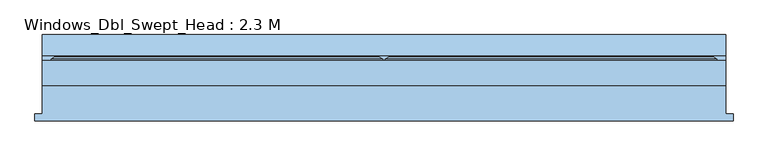
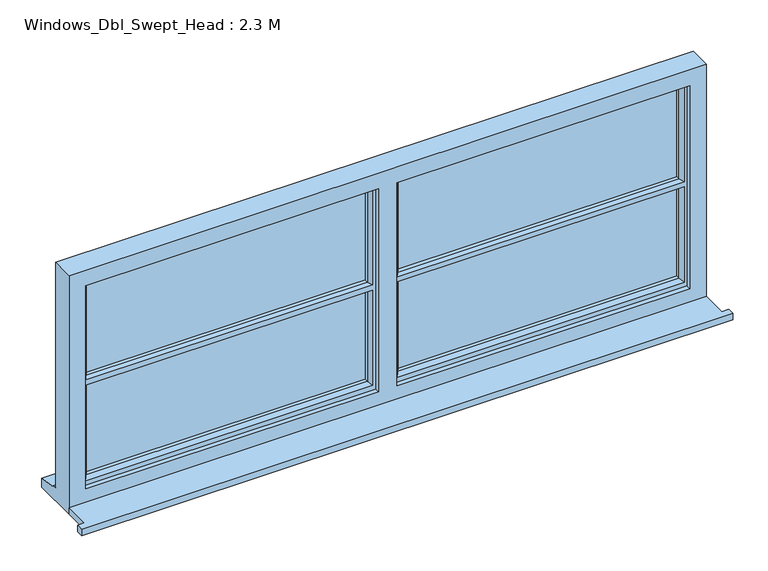
"""IFC4 building model written with IfcOpenShell, lengths in millimetres: window geometry, Windows_Dbl_Swept_Head : 2.3 M."""

from ifc_helpers import new_model, si_unit, frame, origin, place, context, project, spatial, polyline, circle_curve, outline, extrude, faceted_brep, source, transform, mapped, element, save
from ifc_brep_helpers import plane_surface, revolved_surface, advanced_brep


def windows_dbl_swept_head_2_3_m_acbf59cb(model_context):
    return source(origin(), model_context, "Body", "SolidModel", [
        extrude(outline(polyline([(-1460.0, -130.8434322), (-1460.0, -105.8434322), (-1435.0, -105.8434322), (-1435.0, -10.2434322), (865.0, -10.2434322), (865.0, -105.8434322), (890.0, -105.8434322), (890.0, -130.8434322), (-1460.0, -130.8434322)])), frame((0.0, 0.0, 1200.0), z_axis=(0.0, 0.0, 1.0), x_axis=(1.0, 0.0, 0.0)), (0.0, 0.0, 1.0), 25.0),
        extrude(outline(polyline([(795.1480377, 36.7565678), (-240.0, 36.7565678), (-240.0, 60.7565678), (795.1480377, 60.7565678), (795.1480377, 36.7565678)])), frame((0.0, 0.0, 1293.0), z_axis=(0.0, 0.0, 1.0), x_axis=(1.0, 0.0, 0.0)), (0.0, 0.0, 1.0), 365.5),
        extrude(outline(polyline([(795.1480377, 36.7565678), (-240.0, 36.7565678), (-240.0, 60.7565678), (795.1480377, 60.7565678), (795.1480377, 36.7565678)])), frame((0.0, 0.0, 1674.5), z_axis=(0.0, 0.0, 1.0), x_axis=(1.0, 0.0, 0.0)), (0.0, 0.0, 1.0), 365.5),
        extrude(outline(polyline([(-330.0, 36.7565678), (-1365.0, 36.7565678), (-1365.0, 60.7565678), (-330.0, 60.7565678), (-330.0, 36.7565678)])), frame((0.0, 0.0, 1674.5), z_axis=(0.0, 0.0, 1.0), x_axis=(1.0, 0.0, 0.0)), (0.0, 0.0, 1.0), 365.5),
        extrude(outline(polyline([(-330.0, 36.7565678), (-1365.1480377, 36.7565678), (-1365.1480377, 60.7565678), (-330.0, 60.7565678), (-330.0, 36.7565678)])), frame((0.0, 0.0, 1292.8519623), z_axis=(0.0, 0.0, 1.0), x_axis=(1.0, 0.0, 0.0)), (0.0, 0.0, 1.0), 365.6480377),
        faceted_brep([(-1435.0, -10.2434322, 1200.0), (865.0, -10.2434322, 1200.0), (865.0, -10.2434322, 2110.0), (-1435.0, -10.2434322, 2110.0), (-318.0, -10.2434322, 2050.0), (-318.0, -10.2434322, 1275.0), (-1375.0, -10.2434322, 1275.0), (-1375.0, -10.2434322, 2050.0), (-252.0, -10.2434322, 2050.0), (805.0, -10.2434322, 2050.0), (805.0, -10.2434322, 1275.0), (-252.0, -10.2434322, 1275.0), (-1435.0, 72.7565678, 2110.0), (-1435.0, 72.7565678, 1251.0), (-1435.0, 87.7565678, 1249.68767), (-1435.0, 87.7565678, 1244.7449676), (-1435.0, 160.2565678, 1233.8088847), (-1435.0, 160.2565678, 1200.0), (865.0, 72.7565678, 2110.0), (865.0, 72.7565678, 1251.0), (-1395.0, 72.7565678, 2070.0), (-1395.0, 72.7565678, 1263.0), (-300.0, 72.7565678, 1263.0), (-300.0, 72.7565678, 2070.0), (-270.0, 72.7565678, 2070.0), (-270.0, 72.7565678, 1263.0), (825.0, 72.7565678, 1263.0), (825.0, 72.7565678, 2070.0), (-1395.0, 7.7565678, 2070.0), (-1395.0, 7.7565678, 1263.0), (-300.0, 7.7565678, 2070.0), (-300.0, 7.7565678, 1263.0), (-318.0, 7.7565678, 2050.0), (-1375.0, 7.7565678, 2050.0), (-1375.0, 7.7565678, 1275.0), (-318.0, 7.7565678, 1275.0), (-270.0, 7.7565678, 2070.0), (825.0, 7.7565678, 2070.0), (825.0, 7.7565678, 1263.0), (-270.0, 7.7565678, 1263.0), (805.0, 7.7565678, 2050.0), (-252.0, 7.7565678, 2050.0), (-252.0, 7.7565678, 1275.0), (805.0, 7.7565678, 1275.0), (865.0, 160.2565678, 1200.0), (865.0, 160.2565678, 1233.8088847), (865.0, 87.7565678, 1244.7449676), (865.0, 87.7565678, 1249.68767)], [[[0, 1, 2, 3], [4, 5, 6, 7], [8, 9, 10, 11]], [[0, 3, 12, 13, 14, 15, 16, 17]], [[13, 12, 18, 19], [20, 21, 22, 23], [24, 25, 26, 27]], [[21, 20, 28, 29]], [[28, 30, 31, 29], [32, 33, 34, 35]], [[36, 37, 38, 39], [40, 41, 42, 43]], [[33, 7, 6, 34]], [[12, 3, 2, 18]], [[28, 20, 23, 30]], [[27, 37, 36, 24]], [[7, 33, 32, 4]], [[40, 9, 8, 41]], [[19, 18, 2, 1, 44, 45, 46, 47]], [[27, 26, 38, 37]], [[9, 40, 43, 10]], [[23, 22, 31, 30]], [[25, 24, 36, 39]], [[41, 8, 11, 42]], [[4, 32, 35, 5]], [[44, 1, 0, 17]], [[45, 44, 17, 16]], [[46, 45, 16, 15]], [[47, 46, 15, 14]], [[19, 47, 14, 13]], [[22, 21, 29, 31]], [[26, 25, 39, 38]], [[11, 10, 43, 42]], [[35, 34, 6, 5]]]),
        advanced_brep(
        [(-280.0, 72.7565678, 2080.0), (-280.0, 78.5300705, 2080.0), (-280.0, 78.5300705, 1253.0), (-280.0, 72.7565678, 1253.0), (-270.0, 7.7565678, 2070.0), (-270.0, 72.7565678, 2070.0), (-270.0, 72.7565678, 1263.0), (-270.0, 7.7565678, 1263.0), (-230.0, 22.2494677, 2030.0), (-240.1480377, 7.7565678, 2040.1480377), (-240.1480377, 7.7565678, 1676.3519623), (-230.0, 22.2494677, 1681.5), (-240.1480377, 7.7565678, 1292.8519623), (-230.0, 22.2494677, 1303.0), (-230.0, 22.2494677, 1651.5), (-240.1480377, 7.7565678, 1656.6480377), (-230.0, 36.7565678, 2030.0), (-230.0, 36.7565678, 1681.5), (-230.0, 36.7565678, 1303.0), (-230.0, 36.7565678, 1651.5), (-240.0, 60.7565678, 2040.0), (-240.0, 36.7565678, 2040.0), (-240.0, 36.7565678, 1674.5), (-240.0, 60.7565678, 1674.5), (-240.0, 36.7565678, 1293.0), (-240.0, 60.7565678, 1293.0), (-240.0, 60.7565678, 1658.5), (-240.0, 36.7565678, 1658.5), (-230.0, 60.7565678, 1303.0), (-230.0, 78.5300705, 1303.0), (-230.0, 78.5300705, 1651.5), (-230.0, 60.7565678, 1651.5), (-230.0, 60.7565678, 1681.5), (-230.0, 78.5300705, 1681.5), (-230.0, 78.5300705, 1807.124206), (-230.0, 60.7565678, 1807.124206), (-247.4457548, 84.3035732, 2047.4457548), (-230.0, 78.5300705, 2030.0), (-235.0, 80.1847718, 1681.5), (-247.4457548, 84.3035732, 1669.0542452), (-247.4457548, 84.3035732, 1285.5542452), (-247.4457548, 84.3035732, 1663.9457548), (-235.0, 80.1847718, 1651.5), (-269.2153903, 84.3035732, 2069.2153903), (-269.2153903, 84.3035732, 1263.7846097), (835.0, 78.5300705, 1253.0), (835.0, 72.7565678, 1253.0), (825.0, 72.7565678, 1263.0), (825.0, 7.7565678, 1263.0), (795.1480377, 7.7565678, 1292.8519623), (785.0, 22.2494677, 1303.0), (785.0, 36.7565678, 1303.0), (795.0, 36.7565678, 1293.0), (795.0, 60.7565678, 1293.0), (785.0, 60.7565678, 1303.0), (785.0, 78.5300705, 1303.0), (802.4457548, 84.3035732, 1285.5542452), (824.2153903, 84.3035732, 1263.7846097), (835.0, 78.5300705, 2080.0), (835.0, 72.7565678, 2080.0), (825.0, 72.7565678, 2070.0), (825.0, 7.7565678, 2070.0), (795.1480377, 7.7565678, 1656.6480377), (785.0, 22.2494677, 1651.5), (795.1480377, 7.7565678, 2040.1480377), (785.0, 22.2494677, 2030.0), (785.0, 22.2494677, 1681.5), (795.1480377, 7.7565678, 1676.3519623), (785.0, 36.7565678, 1651.5), (785.0, 36.7565678, 2030.0), (785.0, 36.7565678, 1681.5), (795.0, 36.7565678, 1658.5), (795.0, 60.7565678, 1658.5), (795.0, 36.7565678, 2040.0), (795.0, 60.7565678, 2040.0), (795.0, 60.7565678, 1674.5), (795.0, 36.7565678, 1674.5), (785.0, 60.7565678, 1651.5), (785.0, 78.5300705, 1651.5), (785.0, 78.5300705, 1681.5), (785.0, 60.7565678, 1681.5), (785.0, 60.7565678, 1807.124206), (785.0, 78.5300705, 1807.124206), (790.0, 80.1847718, 1651.5), (802.4457548, 84.3035732, 1663.9457548), (785.0, 78.5300705, 2030.0), (802.4457548, 84.3035732, 2047.4457548), (802.4457548, 84.3035732, 1669.0542452), (790.0, 80.1847718, 1681.5), (824.2153903, 84.3035732, 2069.2153903)],
        [
            (0, 1),
            (1, 2),
            (2, 3),
            (3, 0),
            (4, 5),
            (5, 6),
            (6, 7),
            (7, 4),
            (8, 9),
            (9, 10),
            (10, 11),
            (11, 8),
            (12, 13),
            (13, 14),
            (14, 15),
            (15, 12),
            (16, 8),
            (11, 17),
            (17, 16),
            (13, 18),
            (18, 19),
            (19, 14),
            (20, 21),
            (21, 22),
            (22, 23),
            (23, 20),
            (24, 25),
            (25, 26),
            (26, 27),
            (27, 24),
            (28, 29),
            (29, 30),
            (30, 31),
            (31, 28),
            (32, 33),
            (33, 34),
            (34, 35),
            (35, 32),
            (36, 37),
            (37, 34),
            (33, 38),
            (38, 39),
            (39, 36),
            (29, 40),
            (40, 41),
            (41, 42),
            (42, 30),
            (1, 43),
            (43, 44),
            (44, 2),
            (2, 45),
            (45, 46),
            (46, 3),
            (6, 47),
            (47, 48),
            (48, 7),
            (12, 49),
            (49, 50),
            (50, 13),
            (50, 51),
            (51, 18),
            (24, 52),
            (52, 53),
            (53, 25),
            (28, 54),
            (54, 55),
            (55, 29),
            (55, 56),
            (56, 40),
            (44, 57),
            (57, 45),
            (45, 58),
            (58, 59),
            (59, 46),
            (47, 60),
            (60, 61),
            (61, 48),
            (49, 62),
            (62, 63),
            (63, 50),
            (64, 65),
            (65, 66),
            (66, 67),
            (67, 64),
            (63, 68),
            (68, 51),
            (65, 69),
            (69, 70),
            (70, 66),
            (52, 71),
            (71, 72),
            (72, 53),
            (73, 74),
            (74, 75),
            (75, 76),
            (76, 73),
            (54, 77),
            (77, 78),
            (78, 55),
            (79, 80),
            (80, 81),
            (81, 82),
            (82, 79),
            (78, 83),
            (83, 84),
            (84, 56),
            (85, 86),
            (86, 87),
            (87, 88),
            (88, 79),
            (82, 85),
            (57, 89),
            (89, 58),
            (0, 59),
            (58, 1),
            (5, 60),
            (4, 61),
            (15, 62),
            (9, 64),
            (67, 10),
            (8, 65),
            (16, 69),
            (27, 71),
            (68, 19),
            (21, 73),
            (76, 22),
            (17, 70),
            (20, 74),
            (72, 26),
            (31, 77),
            (23, 75),
            (80, 32),
            (35, 81, circle_curve(frame((277.5, 60.7565678, 1325.0), z_axis=(0.0, 1.0, 0.0), x_axis=(1.0, 0.0, 0.0)), 700.0)),
            (36, 86),
            (85, 37),
            (43, 89),
            (84, 41),
            (39, 87),
            (38, 88),
            (11, 66),
            (14, 63),
            (42, 83),
            (82, 34, circle_curve(frame((277.5, 78.5300705, 1325.0), z_axis=(0.0, -1.0, 0.0), x_axis=(1.0, 0.0, 0.0)), 700.0)),
        ],
        [
            plane_surface(frame((-280.0, 78.5300705, 2080.0), z_axis=(-1.0, 0.0, 0.0), x_axis=(0.0, 0.0, -1.0))),
            plane_surface(frame((-270.0, 72.7565678, 2070.0), z_axis=(-1.0, 0.0, 0.0), x_axis=(0.0, 0.0, -1.0))),
            plane_surface(frame((-240.1480377, 7.7565678, 2040.1480377), z_axis=(0.8191520442889492, -0.5735764363511071, 0.0), x_axis=(0.0, 0.0, -1.0))),
            plane_surface(frame((-230.0, 22.2494677, 2030.0), z_axis=(1.0, 0.0, 0.0), x_axis=(0.0, 0.0, -1.0))),
            plane_surface(frame((-240.0, 36.7565678, 2040.0), z_axis=(1.0, 0.0, 0.0), x_axis=(0.0, 0.0, -1.0))),
            plane_surface(frame((-230.0, 60.7565678, 2030.0), z_axis=(1.0, 0.0, 0.0), x_axis=(0.0, 0.0, -1.0))),
            plane_surface(frame((-230.0, 78.5300705, 2030.0), z_axis=(0.31418232948755237, 0.9493626619147053, 0.0), x_axis=(0.0, 0.0, -1.0))),
            plane_surface(frame((-269.2153903, 84.3035732, 2069.2153903), z_axis=(-0.47196942945730275, 0.8816149146071363, 0.0), x_axis=(0.0, 0.0, -1.0))),
            plane_surface(frame((-280.0, 78.5300705, 1253.0), z_axis=(0.0, 0.0, -1.0), x_axis=(1.0, 0.0, 0.0))),
            plane_surface(frame((-270.0, 72.7565678, 1263.0), z_axis=(0.0, 0.0, -1.0), x_axis=(1.0, 0.0, 0.0))),
            plane_surface(frame((-240.1480377, 7.7565678, 1292.8519623), z_axis=(0.0, -0.5735764363511044, 0.819152044288951), x_axis=(1.0, 0.0, 0.0))),
            plane_surface(frame((-230.0, 22.2494677, 1303.0), z_axis=(0.0, 0.0, 1.0), x_axis=(1.0, 0.0, 0.0))),
            plane_surface(frame((-240.0, 36.7565678, 1293.0), z_axis=(0.0, 0.0, 1.0), x_axis=(1.0, 0.0, 0.0))),
            plane_surface(frame((-230.0, 60.7565678, 1303.0), z_axis=(0.0, 0.0, 1.0), x_axis=(1.0, 0.0, 0.0))),
            plane_surface(frame((-230.0, 78.5300705, 1303.0), z_axis=(0.0, 0.9493626619147063, 0.31418232948754926), x_axis=(1.0, 0.0, 0.0))),
            plane_surface(frame((-269.2153903, 84.3035732, 1263.7846097), z_axis=(0.0, 0.8816149146071347, -0.47196942945730563), x_axis=(1.0, 0.0, 0.0))),
            plane_surface(frame((835.0, 78.5300705, 1253.0), z_axis=(1.0, 0.0, 0.0), x_axis=(0.0, 0.0, 1.0))),
            plane_surface(frame((825.0, 72.7565678, 1263.0), z_axis=(1.0, 0.0, 0.0), x_axis=(0.0, 0.0, 1.0))),
            plane_surface(frame((795.1480377, 7.7565678, 1292.8519623), z_axis=(-0.8191520442889529, -0.5735764363511018, 0.0), x_axis=(0.0, 0.0, 1.0))),
            plane_surface(frame((785.0, 22.2494677, 1303.0), z_axis=(-1.0, 0.0, 0.0), x_axis=(0.0, 0.0, 1.0))),
            plane_surface(frame((795.0, 36.7565678, 1293.0), z_axis=(-1.0, 0.0, 0.0), x_axis=(0.0, 0.0, 1.0))),
            plane_surface(frame((785.0, 60.7565678, 1303.0), z_axis=(-1.0, 0.0, 0.0), x_axis=(0.0, 0.0, 1.0))),
            plane_surface(frame((785.0, 78.5300705, 1303.0), z_axis=(-0.3141823294875462, 0.9493626619147074, 0.0), x_axis=(0.0, 0.0, 1.0))),
            plane_surface(frame((824.2153903, 84.3035732, 1263.7846097), z_axis=(0.4719694294573085, 0.8816149146071331, 0.0), x_axis=(0.0, 0.0, 1.0))),
            plane_surface(frame((835.0, 78.5300705, 2080.0), z_axis=(0.0, 0.0, 1.0), x_axis=(-1.0, 0.0, 0.0))),
            plane_surface(frame((835.0, 72.7565678, 2080.0), z_axis=(0.0, -1.0, 0.0), x_axis=(-1.0, 0.0, 0.0))),
            plane_surface(frame((825.0, 72.7565678, 2070.0), z_axis=(0.0, 0.0, 1.0), x_axis=(-1.0, 0.0, 0.0))),
            plane_surface(frame((825.0, 7.7565678, 2070.0), z_axis=(0.0, -1.0, 0.0), x_axis=(-1.0, 0.0, 0.0))),
            plane_surface(frame((795.1480377, 7.7565678, 2040.1480377), z_axis=(0.0, -0.5735764363511044, -0.819152044288951), x_axis=(-1.0, 0.0, 0.0))),
            plane_surface(frame((785.0, 22.2494677, 2030.0), z_axis=(0.0, 0.0, -1.0), x_axis=(-1.0, 0.0, 0.0))),
            plane_surface(frame((785.0, 36.7565678, 2030.0), z_axis=(0.0, 1.0, 0.0), x_axis=(-1.0, 0.0, 0.0))),
            plane_surface(frame((795.0, 36.7565678, 2040.0), z_axis=(0.0, 0.0, -1.0), x_axis=(-1.0, 0.0, 0.0))),
            plane_surface(frame((795.0, 60.7565678, 2040.0), z_axis=(0.0, -1.0, 0.0), x_axis=(-1.0, 0.0, 0.0))),
            plane_surface(frame((785.0, 78.5300705, 2030.0), z_axis=(0.0, 0.9493626619147064, -0.3141823294875493), x_axis=(-1.0, 0.0, 0.0))),
            plane_surface(frame((802.4457548, 84.3035732, 2047.4457548), z_axis=(0.0, 1.0, 0.0), x_axis=(-1.0, 0.0, 0.0))),
            plane_surface(frame((824.2153903, 84.3035732, 2069.2153903), z_axis=(0.0, 0.8816149146071347, 0.47196942945730563), x_axis=(-1.0, 0.0, 0.0))),
            plane_surface(frame((802.4457548, 84.3035732, 1669.0542452), z_axis=(0.0, 0.9493626619145938, 0.3141823294878896), x_axis=(-1.0, 0.0, 0.0))),
            plane_surface(frame((802.4457548, 80.1847718, 1681.5), z_axis=(0.0, 0.0, 1.0), x_axis=(-1.0, 0.0, 0.0))),
            plane_surface(frame((802.4457548, 60.7565678, 1674.5), z_axis=(0.0, 0.0, 1.0), x_axis=(-1.0, 0.0, 0.0))),
            plane_surface(frame((802.4457548, 36.7565678, 1681.5), z_axis=(0.0, 0.0, 1.0), x_axis=(-1.0, 0.0, 0.0))),
            plane_surface(frame((802.4457548, 22.2494677, 1681.5), z_axis=(0.0, -0.33472142672711697, 0.9423171262848634), x_axis=(-1.0, 0.0, 0.0))),
            plane_surface(frame((802.4457548, 7.7565678, 1656.6480377), z_axis=(0.0, -0.33472142672499106, -0.9423171262856186), x_axis=(-1.0, 0.0, 0.0))),
            plane_surface(frame((802.4457548, 22.2494677, 1651.5), z_axis=(0.0, 0.0, -1.0), x_axis=(-1.0, 0.0, 0.0))),
            plane_surface(frame((802.4457548, 36.7565678, 1658.5), z_axis=(0.0, 0.0, -1.0), x_axis=(-1.0, 0.0, 0.0))),
            plane_surface(frame((802.4457548, 60.7565678, 1651.5), z_axis=(0.0, 0.0, -1.0), x_axis=(-1.0, 0.0, 0.0))),
            plane_surface(frame((802.4457548, 80.1847718, 1651.5), z_axis=(0.0, 0.9493626619148547, -0.31418232948710106), x_axis=(-1.0, 0.0, 0.0))),
            plane_surface(frame((-230.0, 78.5300705, 2030.0), z_axis=(0.0, 1.0, 0.0), x_axis=(0.0, 0.0, 1.0))),
            revolved_surface(polyline([(977.5, 78.5300705, 1325.0), (977.5, 60.7565678, 1325.0)]), (277.5, 78.5300705, 1325.0), (0.0, 1.0, 0.0)),
        ],
        [
            (0, [[1, 2, 3, 4]]),
            (1, [[5, 6, 7, 8]]),
            (2, [[9, 10, 11, 12]]),
            (2, [[13, 14, 15, 16]]),
            (3, [[17, -12, 18, 19]]),
            (3, [[20, 21, 22, -14]]),
            (4, [[23, 24, 25, 26]]),
            (4, [[27, 28, 29, 30]]),
            (5, [[31, 32, 33, 34]]),
            (5, [[35, 36, 37, 38]]),
            (6, [[39, 40, -36, 41, 42, 43]]),
            (6, [[44, 45, 46, 47, -32]]),
            (7, [[-2, 48, 49, 50]]),
            (8, [[-3, 51, 52, 53]]),
            (9, [[-7, 54, 55, 56]]),
            (10, [[-13, 57, 58, 59]]),
            (11, [[-20, -59, 60, 61]]),
            (12, [[-27, 62, 63, 64]]),
            (13, [[-31, 65, 66, 67]]),
            (14, [[-44, -67, 68, 69]]),
            (15, [[-50, 70, 71, -51]]),
            (16, [[-52, 72, 73, 74]]),
            (17, [[-55, 75, 76, 77]]),
            (18, [[-58, 78, 79, 80]]),
            (18, [[81, 82, 83, 84]]),
            (19, [[-60, -80, 85, 86]]),
            (19, [[87, 88, 89, -82]]),
            (20, [[-63, 90, 91, 92]]),
            (20, [[93, 94, 95, 96]]),
            (21, [[-66, 97, 98, 99]]),
            (21, [[100, 101, 102, 103]]),
            (22, [[-68, -99, 104, 105, 106]]),
            (22, [[107, 108, 109, 110, -103, 111]]),
            (23, [[-71, 112, 113, -72]]),
            (24, [[-1, 114, -73, 115]]),
            (25, [[-4, -53, -74, -114], [-6, 116, -75, -54]]),
            (26, [[-5, 117, -76, -116]]),
            (27, [[-8, -56, -77, -117], [-57, -16, 118, -78], [119, -84, 120, -10]]),
            (28, [[-9, 121, -81, -119]]),
            (29, [[-17, 122, -87, -121]]),
            (30, [[-62, -30, 123, -90], [-61, -86, 124, -21]]),
            (30, [[125, -96, 126, -24], [-122, -19, 127, -88]]),
            (31, [[-23, 128, -93, -125]]),
            (32, [[-64, -92, 129, -28], [-65, -34, 130, -97]]),
            (32, [[-128, -26, 131, -94], [132, -38, 133, -101]]),
            (33, [[-39, 134, -107, 135]]),
            (34, [[-49, 136, -112, -70], [-69, -106, 137, -45], [-134, -43, 138, -108]]),
            (35, [[-48, -115, -113, -136]]),
            (36, [[-138, -42, 139, -109]]),
            (37, [[-132, -100, -110, -139, -41, -35]]),
            (38, [[-25, -126, -95, -131]]),
            (39, [[140, -89, -127, -18]]),
            (40, [[-120, -83, -140, -11]]),
            (41, [[-118, -15, 141, -79]]),
            (42, [[-141, -22, -124, -85]]),
            (43, [[-29, -129, -91, -123]]),
            (44, [[-130, -33, -47, 142, -104, -98]]),
            (45, [[-137, -105, -142, -46]]),
            (46, [[143, -40, -135, -111]]),
            (47, [[-133, -37, -143, -102]]),
        ],
    ),
        advanced_brep(
        [(-330.0, 60.7565678, 2040.0), (-1365.0, 60.7565678, 2040.0), (-1365.0, 60.7565678, 1674.5), (-330.0, 60.7565678, 1674.5), (-1355.0, 60.7565678, 1807.124206), (-340.0, 60.7565678, 1807.124206), (-340.0, 60.7565678, 1681.5), (-1355.0, 60.7565678, 1681.5), (-1365.0, 60.7565678, 1293.0), (-330.0, 60.7565678, 1293.0), (-330.0, 60.7565678, 1658.5), (-1365.0, 60.7565678, 1658.5), (-340.0, 60.7565678, 1303.0), (-1355.0, 60.7565678, 1303.0), (-1355.0, 60.7565678, 1651.5), (-340.0, 60.7565678, 1651.5), (-1405.0, 72.7565678, 2080.0), (-1405.0, 78.5300705, 2080.0), (-1405.0, 78.5300705, 1253.0), (-1405.0, 72.7565678, 1253.0), (-1395.0, 7.7565678, 2070.0), (-1395.0, 72.7565678, 2070.0), (-1395.0, 72.7565678, 1263.0), (-1395.0, 7.7565678, 1263.0), (-1355.0, 22.2494677, 2030.0), (-1365.1480377, 7.7565678, 2040.1480377), (-1365.1480377, 7.7565678, 1676.3519623), (-1355.0, 22.2494677, 1681.5), (-1365.1480377, 7.7565678, 1292.8519623), (-1355.0, 22.2494677, 1303.0), (-1355.0, 22.2494677, 1651.5), (-1365.1480377, 7.7565678, 1656.6480377), (-1355.0, 36.7565678, 2030.0), (-1355.0, 36.7565678, 1681.5), (-1355.0, 36.7565678, 1303.0), (-1355.0, 36.7565678, 1651.5), (-1365.0, 36.7565678, 2040.0), (-1365.0, 36.7565678, 1674.5), (-1365.0, 36.7565678, 1293.0), (-1365.0, 36.7565678, 1658.5), (-1355.0, 78.5300705, 1303.0), (-1355.0, 78.5300705, 1651.5), (-1355.0, 78.5300705, 1681.5), (-1355.0, 78.5300705, 1807.124206), (-1372.4457548, 84.3035732, 2047.4457548), (-1355.0, 78.5300705, 2030.0), (-1360.0, 80.1847718, 1681.5), (-1372.4457548, 84.3035732, 1669.0542452), (-1372.4457548, 84.3035732, 1285.5542452), (-1372.4457548, 84.3035732, 1663.9457548), (-1360.0, 80.1847718, 1651.5), (-1394.2153903, 84.3035732, 2069.2153903), (-1394.2153903, 84.3035732, 1263.7846097), (-290.0, 78.5300705, 1253.0), (-290.0, 72.7565678, 1253.0), (-300.0, 72.7565678, 1263.0), (-300.0, 7.7565678, 1263.0), (-329.8519623, 7.7565678, 1292.8519623), (-340.0, 22.2494677, 1303.0), (-340.0, 36.7565678, 1303.0), (-330.0, 36.7565678, 1293.0), (-340.0, 78.5300705, 1303.0), (-322.5542452, 84.3035732, 1285.5542452), (-300.7846097, 84.3035732, 1263.7846097), (-290.0, 78.5300705, 2080.0), (-290.0, 72.7565678, 2080.0), (-300.0, 72.7565678, 2070.0), (-300.0, 7.7565678, 2070.0), (-329.8519623, 7.7565678, 1656.6480377), (-340.0, 22.2494677, 1651.5), (-329.8519623, 7.7565678, 2040.1480377), (-340.0, 22.2494677, 2030.0), (-340.0, 22.2494677, 1681.5), (-329.8519623, 7.7565678, 1676.3519623), (-340.0, 36.7565678, 1651.5), (-340.0, 36.7565678, 2030.0), (-340.0, 36.7565678, 1681.5), (-330.0, 36.7565678, 1658.5), (-330.0, 36.7565678, 2040.0), (-330.0, 36.7565678, 1674.5), (-340.0, 78.5300705, 1651.5), (-340.0, 78.5300705, 1681.5), (-340.0, 78.5300705, 1807.124206), (-335.0, 80.1847718, 1651.5), (-322.5542452, 84.3035732, 1663.9457548), (-340.0, 78.5300705, 2030.0), (-322.5542452, 84.3035732, 2047.4457548), (-322.5542452, 84.3035732, 1669.0542452), (-335.0, 80.1847718, 1681.5), (-300.7846097, 84.3035732, 2069.2153903)],
        [
            (0, 1),
            (1, 2),
            (2, 3),
            (3, 0),
            (4, 5, circle_curve(frame((-847.5, 60.7565678, 1325.0), z_axis=(0.0, 1.0, 0.0), x_axis=(1.0, 0.0, 0.0)), 700.0)),
            (5, 6),
            (6, 7),
            (7, 4),
            (8, 9),
            (9, 10),
            (10, 11),
            (11, 8),
            (12, 13),
            (13, 14),
            (14, 15),
            (15, 12),
            (16, 17),
            (17, 18),
            (18, 19),
            (19, 16),
            (20, 21),
            (21, 22),
            (22, 23),
            (23, 20),
            (24, 25),
            (25, 26),
            (26, 27),
            (27, 24),
            (28, 29),
            (29, 30),
            (30, 31),
            (31, 28),
            (32, 24),
            (27, 33),
            (33, 32),
            (29, 34),
            (34, 35),
            (35, 30),
            (1, 36),
            (36, 37),
            (37, 2),
            (38, 8),
            (11, 39),
            (39, 38),
            (13, 40),
            (40, 41),
            (41, 14),
            (7, 42),
            (42, 43),
            (43, 4),
            (44, 45),
            (45, 43),
            (42, 46),
            (46, 47),
            (47, 44),
            (40, 48),
            (48, 49),
            (49, 50),
            (50, 41),
            (17, 51),
            (51, 52),
            (52, 18),
            (18, 53),
            (53, 54),
            (54, 19),
            (22, 55),
            (55, 56),
            (56, 23),
            (28, 57),
            (57, 58),
            (58, 29),
            (58, 59),
            (59, 34),
            (38, 60),
            (60, 9),
            (12, 61),
            (61, 40),
            (61, 62),
            (62, 48),
            (52, 63),
            (63, 53),
            (53, 64),
            (64, 65),
            (65, 54),
            (55, 66),
            (66, 67),
            (67, 56),
            (57, 68),
            (68, 69),
            (69, 58),
            (70, 71),
            (71, 72),
            (72, 73),
            (73, 70),
            (69, 74),
            (74, 59),
            (71, 75),
            (75, 76),
            (76, 72),
            (60, 77),
            (77, 10),
            (78, 0),
            (3, 79),
            (79, 78),
            (15, 80),
            (80, 61),
            (81, 6),
            (5, 82),
            (82, 81),
            (80, 83),
            (83, 84),
            (84, 62),
            (85, 86),
            (86, 87),
            (87, 88),
            (88, 81),
            (82, 85),
            (63, 89),
            (89, 64),
            (16, 65),
            (64, 17),
            (21, 66),
            (20, 67),
            (31, 68),
            (25, 70),
            (73, 26),
            (24, 71),
            (32, 75),
            (39, 77),
            (74, 35),
            (36, 78),
            (79, 37),
            (33, 76),
            (44, 86),
            (85, 45),
            (51, 89),
            (84, 49),
            (47, 87),
            (46, 88),
            (83, 50),
            (69, 30),
            (72, 27),
            (82, 43, circle_curve(frame((-847.5, 78.5300705, 1325.0), z_axis=(0.0, -1.0, 0.0), x_axis=(1.0, 0.0, 0.0)), 700.0)),
        ],
        [
            plane_surface(frame((795.0, 60.7565678, 2040.0), z_axis=(0.0, -1.0, 0.0), x_axis=(-1.0, 0.0, 0.0))),
            plane_surface(frame((-1405.0, 78.5300705, 2080.0), z_axis=(-1.0, 0.0, 0.0), x_axis=(0.0, 0.0, -1.0))),
            plane_surface(frame((-1395.0, 72.7565678, 2070.0), z_axis=(-1.0, 0.0, 0.0), x_axis=(0.0, 0.0, -1.0))),
            plane_surface(frame((-1365.1480377, 7.7565678, 2040.1480377), z_axis=(0.8191520442889492, -0.5735764363511071, 0.0), x_axis=(0.0, 0.0, -1.0))),
            plane_surface(frame((-1355.0, 22.2494677, 2030.0), z_axis=(1.0, 0.0, 0.0), x_axis=(0.0, 0.0, -1.0))),
            plane_surface(frame((-1365.0, 36.7565678, 2040.0), z_axis=(1.0, 0.0, 0.0), x_axis=(0.0, 0.0, -1.0))),
            plane_surface(frame((-1355.0, 60.7565678, 2030.0), z_axis=(1.0, 0.0, 0.0), x_axis=(0.0, 0.0, -1.0))),
            plane_surface(frame((-1355.0, 78.5300705, 2030.0), z_axis=(0.31418232948755237, 0.9493626619147053, 0.0), x_axis=(0.0, 0.0, -1.0))),
            plane_surface(frame((-1394.2153903, 84.3035732, 2069.2153903), z_axis=(-0.47196942945730275, 0.8816149146071363, 0.0), x_axis=(0.0, 0.0, -1.0))),
            plane_surface(frame((-1405.0, 78.5300705, 1253.0), z_axis=(0.0, 0.0, -1.0), x_axis=(1.0, 0.0, 0.0))),
            plane_surface(frame((-1395.0, 72.7565678, 1263.0), z_axis=(0.0, 0.0, -1.0), x_axis=(1.0, 0.0, 0.0))),
            plane_surface(frame((-1365.1480377, 7.7565678, 1292.8519623), z_axis=(0.0, -0.5735764363511044, 0.819152044288951), x_axis=(1.0, 0.0, 0.0))),
            plane_surface(frame((-1355.0, 22.2494677, 1303.0), z_axis=(0.0, 0.0, 1.0), x_axis=(1.0, 0.0, 0.0))),
            plane_surface(frame((-1365.0, 36.7565678, 1293.0), z_axis=(0.0, 0.0, 1.0), x_axis=(1.0, 0.0, 0.0))),
            plane_surface(frame((-1355.0, 60.7565678, 1303.0), z_axis=(0.0, 0.0, 1.0), x_axis=(1.0, 0.0, 0.0))),
            plane_surface(frame((-1355.0, 78.5300705, 1303.0), z_axis=(0.0, 0.9493626619147063, 0.31418232948754926), x_axis=(1.0, 0.0, 0.0))),
            plane_surface(frame((-1394.2153903, 84.3035732, 1263.7846097), z_axis=(0.0, 0.8816149146071347, -0.47196942945730563), x_axis=(1.0, 0.0, 0.0))),
            plane_surface(frame((-290.0, 78.5300705, 1253.0), z_axis=(1.0, 0.0, 0.0), x_axis=(0.0, 0.0, 1.0))),
            plane_surface(frame((-300.0, 72.7565678, 1263.0), z_axis=(1.0, 0.0, 0.0), x_axis=(0.0, 0.0, 1.0))),
            plane_surface(frame((-329.8519623, 7.7565678, 1292.8519623), z_axis=(-0.8191520442889529, -0.5735764363511018, 0.0), x_axis=(0.0, 0.0, 1.0))),
            plane_surface(frame((-340.0, 22.2494677, 1303.0), z_axis=(-1.0, 0.0, 0.0), x_axis=(0.0, 0.0, 1.0))),
            plane_surface(frame((-330.0, 36.7565678, 1293.0), z_axis=(-1.0, 0.0, 0.0), x_axis=(0.0, 0.0, 1.0))),
            plane_surface(frame((-340.0, 60.7565678, 1303.0), z_axis=(-1.0, 0.0, 0.0), x_axis=(0.0, 0.0, 1.0))),
            plane_surface(frame((-340.0, 78.5300705, 1303.0), z_axis=(-0.3141823294875462, 0.9493626619147074, 0.0), x_axis=(0.0, 0.0, 1.0))),
            plane_surface(frame((-300.7846097, 84.3035732, 1263.7846097), z_axis=(0.4719694294573085, 0.8816149146071331, 0.0), x_axis=(0.0, 0.0, 1.0))),
            plane_surface(frame((-290.0, 78.5300705, 2080.0), z_axis=(0.0, 0.0, 1.0), x_axis=(-1.0, 0.0, 0.0))),
            plane_surface(frame((-290.0, 72.7565678, 2080.0), z_axis=(0.0, -1.0, 0.0), x_axis=(-1.0, 0.0, 0.0))),
            plane_surface(frame((-300.0, 72.7565678, 2070.0), z_axis=(0.0, 0.0, 1.0), x_axis=(-1.0, 0.0, 0.0))),
            plane_surface(frame((-300.0, 7.7565678, 2070.0), z_axis=(0.0, -1.0, 0.0), x_axis=(-1.0, 0.0, 0.0))),
            plane_surface(frame((-329.8519623, 7.7565678, 2040.1480377), z_axis=(0.0, -0.5735764363511044, -0.819152044288951), x_axis=(-1.0, 0.0, 0.0))),
            plane_surface(frame((-340.0, 22.2494677, 2030.0), z_axis=(0.0, 0.0, -1.0), x_axis=(-1.0, 0.0, 0.0))),
            plane_surface(frame((-340.0, 36.7565678, 2030.0), z_axis=(0.0, 1.0, 0.0), x_axis=(-1.0, 0.0, 0.0))),
            plane_surface(frame((-330.0, 36.7565678, 2040.0), z_axis=(0.0, 0.0, -1.0), x_axis=(-1.0, 0.0, 0.0))),
            plane_surface(frame((-340.0, 78.5300705, 2030.0), z_axis=(0.0, 0.9493626619147064, -0.3141823294875493), x_axis=(-1.0, 0.0, 0.0))),
            plane_surface(frame((-322.5542452, 84.3035732, 2047.4457548), z_axis=(0.0, 1.0, 0.0), x_axis=(-1.0, 0.0, 0.0))),
            plane_surface(frame((-300.7846097, 84.3035732, 2069.2153903), z_axis=(0.0, 0.8816149146071347, 0.47196942945730563), x_axis=(-1.0, 0.0, 0.0))),
            plane_surface(frame((-1372.4457548, 80.1847718, 1681.5), z_axis=(0.0, 0.9493626619144715, 0.31418232948825914), x_axis=(1.0, 0.0, 0.0))),
            plane_surface(frame((-1372.4457548, 84.3035732, 1663.9457548), z_axis=(0.0, 0.949362661914977, -0.3141823294867314), x_axis=(1.0, 0.0, 0.0))),
            plane_surface(frame((-1372.4457548, 80.1847718, 1651.5), z_axis=(0.0, 0.0, -1.0), x_axis=(1.0, 0.0, 0.0))),
            plane_surface(frame((-1372.4457548, 60.7565678, 1658.5), z_axis=(0.0, 0.0, -1.0), x_axis=(1.0, 0.0, 0.0))),
            plane_surface(frame((-1372.4457548, 36.7565678, 1651.5), z_axis=(0.0, 0.0, -1.0), x_axis=(1.0, 0.0, 0.0))),
            plane_surface(frame((-1372.4457548, 22.2494677, 1651.5), z_axis=(0.0, -0.3347214267259168, -0.9423171262852897), x_axis=(1.0, 0.0, 0.0))),
            plane_surface(frame((-1372.4457548, 7.7565678, 1676.3519623), z_axis=(0.0, -0.33472142672616695, 0.9423171262852009), x_axis=(1.0, 0.0, 0.0))),
            plane_surface(frame((-1372.4457548, 22.2494677, 1681.5), z_axis=(0.0, 0.0, 1.0), x_axis=(1.0, 0.0, 0.0))),
            plane_surface(frame((-1372.4457548, 36.7565678, 1674.5), z_axis=(0.0, 0.0, 1.0), x_axis=(1.0, 0.0, 0.0))),
            plane_surface(frame((-1372.4457548, 60.7565678, 1681.5), z_axis=(0.0, 0.0, 1.0), x_axis=(1.0, 0.0, 0.0))),
            plane_surface(frame((-230.0, 78.5300705, 2030.0), z_axis=(0.0, 1.0, 0.0), x_axis=(0.0, 0.0, 1.0))),
            revolved_surface(polyline([(-147.5, 78.5300705, 1325.0), (-147.5, 60.7565678, 1325.0)]), (-847.5, 72.7565678, 1325.0), (0.0, 1.0, 0.0)),
        ],
        [
            (0, [[1, 2, 3, 4], [5, 6, 7, 8]]),
            (0, [[9, 10, 11, 12], [13, 14, 15, 16]]),
            (1, [[17, 18, 19, 20]]),
            (2, [[21, 22, 23, 24]]),
            (3, [[25, 26, 27, 28]]),
            (3, [[29, 30, 31, 32]]),
            (4, [[33, -28, 34, 35]]),
            (4, [[36, 37, 38, -30]]),
            (5, [[39, 40, 41, -2]]),
            (5, [[42, -12, 43, 44]]),
            (6, [[45, 46, 47, -14]]),
            (6, [[48, 49, 50, -8]]),
            (7, [[51, 52, -49, 53, 54, 55]]),
            (7, [[56, 57, 58, 59, -46]]),
            (8, [[-18, 60, 61, 62]]),
            (9, [[-19, 63, 64, 65]]),
            (10, [[-23, 66, 67, 68]]),
            (11, [[-29, 69, 70, 71]]),
            (12, [[-36, -71, 72, 73]]),
            (13, [[-42, 74, 75, -9]]),
            (14, [[-45, -13, 76, 77]]),
            (15, [[-56, -77, 78, 79]]),
            (16, [[-62, 80, 81, -63]]),
            (17, [[-64, 82, 83, 84]]),
            (18, [[-67, 85, 86, 87]]),
            (19, [[-70, 88, 89, 90]]),
            (19, [[91, 92, 93, 94]]),
            (20, [[-72, -90, 95, 96]]),
            (20, [[97, 98, 99, -92]]),
            (21, [[-75, 100, 101, -10]]),
            (21, [[102, -4, 103, 104]]),
            (22, [[-76, -16, 105, 106]]),
            (22, [[107, -6, 108, 109]]),
            (23, [[-78, -106, 110, 111, 112]]),
            (23, [[113, 114, 115, 116, -109, 117]]),
            (24, [[-81, 118, 119, -82]]),
            (25, [[-17, 120, -83, 121]]),
            (26, [[-20, -65, -84, -120], [-22, 122, -85, -66]]),
            (27, [[-21, 123, -86, -122]]),
            (28, [[-24, -68, -87, -123], [-69, -32, 124, -88], [125, -94, 126, -26]]),
            (29, [[-25, 127, -91, -125]]),
            (30, [[-33, 128, -97, -127]]),
            (31, [[-74, -44, 129, -100], [-73, -96, 130, -37]]),
            (31, [[131, -104, 132, -40], [-128, -35, 133, -98]]),
            (32, [[-39, -1, -102, -131]]),
            (33, [[-51, 134, -113, 135]]),
            (34, [[-61, 136, -118, -80], [-79, -112, 137, -57], [-134, -55, 138, -114]]),
            (35, [[-60, -121, -119, -136]]),
            (36, [[-138, -54, 139, -115]]),
            (37, [[-137, -111, 140, -58]]),
            (38, [[-15, -47, -59, -140, -110, -105]]),
            (39, [[-43, -11, -101, -129]]),
            (40, [[141, -38, -130, -95]]),
            (41, [[-124, -31, -141, -89]]),
            (42, [[-126, -93, 142, -27]]),
            (43, [[-142, -99, -133, -34]]),
            (44, [[-41, -132, -103, -3]]),
            (45, [[-7, -107, -116, -139, -53, -48]]),
            (46, [[143, -52, -135, -117]]),
            (47, [[-5, -50, -143, -108]]),
        ],
    ),
    ])


if __name__ == "__main__":
    model = new_model("IFC4")
    model_context = context("Model", 3, world=origin())
    ifc_project = project(units=[si_unit("LENGTHUNIT", "METRE", prefix="MILLI")], contexts=[model_context])
    site = spatial("IfcSite", under=ifc_project)
    building = spatial("IfcBuilding", under=site)
    placement = place(None, origin())
    windows_dbl_swept_head_2_3_m_shape = windows_dbl_swept_head_2_3_m_acbf59cb(model_context)
    element("IfcWindow", 1, ObjectType="Windows_Dbl_Swept_Head : 2.3 M", at=placement, inside=building, context=model_context, shape_type="MappedRepresentation", body=[
        mapped(windows_dbl_swept_head_2_3_m_shape, transform((0.0, 0.0, 0.0), x_axis=(1.0, 0.0, 0.0), y_axis=(0.0, 1.0, 0.0), z_axis=(0.0, 0.0, 1.0))),
    ])
    save(model, "model.ifc")

# Revit data of these elements
# Type "Windows_Dbl_Swept_Head : 2.3 M"
#   Type Mark = "69"
#   Operation = "DoublePanelVertical"
#   Construction Type Id = "GSP4R"
#   Manufacturer = "Revit"
#   Keynote = "L10"
#   Analytic Construction = "1/8 in Pilkington single glazing"
#   Wrap Layers (Ext) from Ext = 0.1025 m
#   Wrap Layers (Int) from Ext = 0.1775 m
#   Window Board Projection = 0.025 m
#   Window Board Extension = 0.025 m
#   Visual Light Transmittance = 0.9
#   Solar Heat Gain Coefficient = 0.78
#   Rough Width = 2.3 m
#   Rough Height = 0.91 m
#   Radius - Swept Head = 0.7 m
#   Height = 0.91 m
#   Width = 2.3 m
#   Heat Transfer Coefficient (U) = 3.6886 W/(m²·K)
#   Glazing Thickness = 0.024 m
#   FrameOffset - External = 0.05 m
#   Frame Depth = 0.065 m
#   Default Head Height = 2.11 m
#   Cill Depth = 0.0875 m
#   Cavity Closer Width = 0.05 m
#   Cavity Closer Offset from Ext = 0.1025 m
#   Cavity Closer Depth = 0.085 m
#   Vis - Cavity Closers = yes
#   Define Thermal Properties by = 1
#   Material Trim = Window Frame
#   Material Glass = Glass
#   Material Frame = Window Frame
#   Wall Closure = (empty or 0)
# Element 1 (IfcWindow, "Windows_Dbl_Swept_Head : 2.3 M")
#   Materials on its faces: "Window Frame", "Glass"
# Materials
#   "Window Frame": colour RGB 249 249 249, transparency 0, Keynote = "L10", Cost = 0
#   "Glass": class "Glass", colour RGB 0 128 192, transparency 0.9, Description = "Soda Lime Glass", Cost = 0
